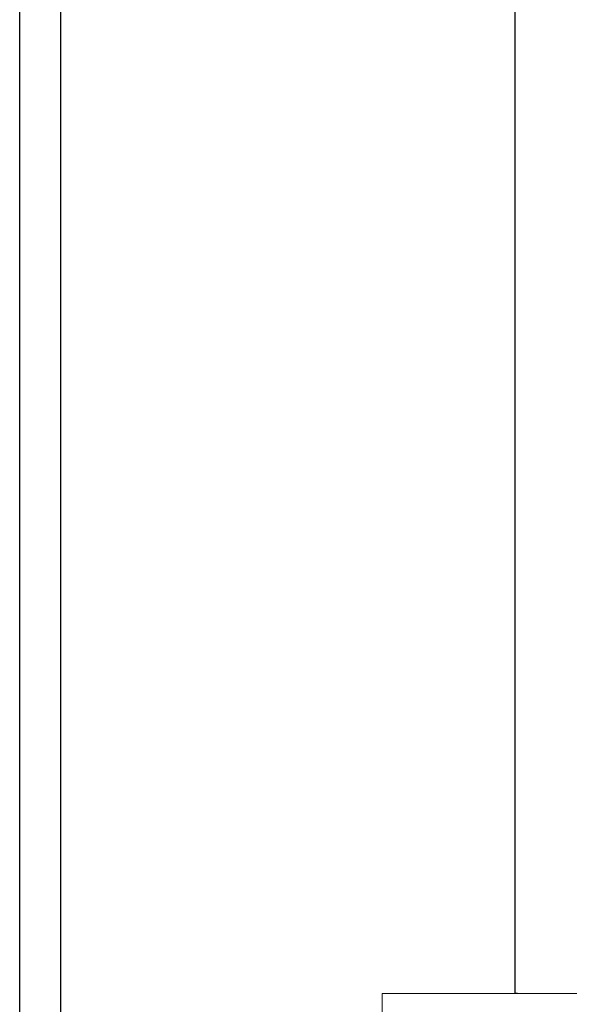
# Model space of a CAD drawing. Units: inches. Extents: x 0 to 4258, y 0 to 3769.
# Tile 2 of 30: x 3476 to 3659, y 2933 to 3261. Entities that reach past the tile are written whole.
import ezdxf

# ---------------------------------------------------------------- set-up
doc = ezdxf.new("R2010")
doc.units = ezdxf.units.IN
doc.header["$MEASUREMENT"] = 0
for name, color, linetype, lineweight in [('A-ANNO-DIMS', 250, 'Continuous', 18), ('A-ANNO-TTLB', 250, 'Continuous', 25), ('C-ROAD', 250, 'Continuous', 18)]:
    doc.layers.add(name, color=color, linetype=linetype, lineweight=lineweight)
doc.styles.get("Standard").update_dxf_attribs({"font": 'arial.ttf'})
doc.dimstyles.get("Standard").update_dxf_attribs({"dimtxt": 7, "dimasz": 0.18, "dimexe": 0.18, "dimexo": 0.0625, "dimgap": 0.09, "dimtad": 0, "dimtih": 1, "dimtoh": 1, "dimzin": 0, "dimdsep": 46, "dimlunit": 3, "dimtxsty": 'Standard', "dimcen": 0.09, "dimadec": 0, "dimazin": 0, "dimtfac": 1, "dimtofl": 0, "dimtmove": 0, "dimatfit": 3, "dimfxl": 1, "dimtolj": 1, "dimtzin": 0, "dimarcsym": 0})

# ---------------------------------------------------------------- blocks, each defined once
blk = doc.blocks.new('*D25')
at = {"layer": 'A-ANNO-DIMS', "color": 0, "lineweight": -2, "transparency": 16777216}
for p, q in [((3641.78, 3656.79), (3640.81, 3656.79)), ((3640.99, 3656.61), (3640.99, 3300.46)), ((3640.99, 2936.97), (3640.99, 3293.13)), ((3641.78, 2936.79), (3640.81, 2936.79))]:
    blk.add_line(p, q, dxfattribs=at)
at = {"layer": 'A-ANNO-DIMS', "color": 0, "transparency": 16777216}
for points in [[(3640.96, 3656.61), (3641.02, 3656.61), (3640.99, 3656.79)], [(3640.96, 2936.97), (3641.02, 2936.97), (3640.99, 2936.79)]]:
    blk.add_solid(points, dxfattribs=at)
at = {"layer": 'Defpoints', "color": 0, "transparency": 16777216}
for p in [(3641.85, 3656.79), (3640.99, 2936.79), (3641.85, 2936.79)]:
    blk.add_point(p, dxfattribs=at)
at = {"layer": 'A-ANNO-DIMS', "color": 0, "transparency": 16777216, "insert": (3640.99, 3296.79), "char_height": 7, "attachment_point": 5}
blk.add_mtext("\\A1;60'", dxfattribs=at)

msp = doc.modelspace()

# ---------------------------------------------------------------- linework, layer by layer
at = {"layer": 'A-ANNO-TTLB'}
for p, q in [((3476.156, 2762.335), (3476.156, 3768.679)), ((3489.722, 3758.41), (3489.722, 2762.335))]:
    msp.add_line(p, q, dxfattribs=at)
at = {"layer": 'C-ROAD'}
for p, q in [((3678.804, 2936.793), (3596.728, 2936.793)), ((3596.728, 2936.793), (3596.728, 2860.957))]:
    msp.add_line(p, q, dxfattribs=at)

# ---------------------------------------------------------------- dimensions: what is measured, and where the dimension line sits
at = {"layer": 'A-ANNO-DIMS'}
dim = msp.add_linear_dim(base=(3640.987, 2936.793), p1=(3641.847, 3656.793), p2=(3641.847, 2936.793), angle=90, dimstyle='Standard', override={"dimclrd": 0, "dimclre": 0, "dimclrt": 0}, dxfattribs=at)
dim.commit()
dim.dimension.update_dxf_attribs({"geometry": '*D25', "text_midpoint": (3640.987, 3296.793)})

doc.saveas('drawing.dxf')
